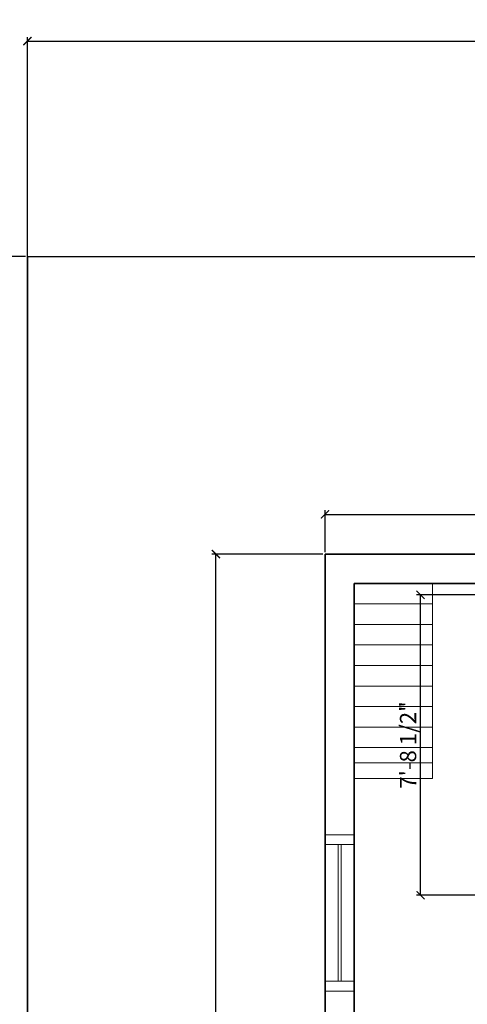
# Model space of a CAD drawing. Units: inches. Extents: x 3283068 to 3284536, y 3240756 to 3241803.
# Tile 8 of 19: x 3283246 to 3283383, y 3241501 to 3241803. Entities that reach past the tile are written whole.
import ezdxf

# ---------------------------------------------------------------- set-up
doc = ezdxf.new("R2010")
doc.units = ezdxf.units.IN
for name, color, linetype, lineweight in [('A-ANNO-DIMS', 2, 'Continuous', 18), ('C-PROP', 7, 'Continuous', 25), ('wall', 20, 'Continuous', 35), ('wardrobe', 180, 'Continuous', 18), ('window', 100, 'Continuous', 18)]:
    doc.layers.add(name, color=color, linetype=linetype, lineweight=lineweight)
doc.styles.get("Standard").update_dxf_attribs({"font": 'arial.ttf'})
doc.dimstyles.new('ISO-25', dxfattribs={"dimtxt": 5, "dimasz": 2.5, "dimexe": 1.25, "dimexo": 0.625, "dimtad": 1, "dimlunit": 4, "dimtxsty": 'Standard', "dimblk": 'ARCHTICK', "dimcen": 2.5, "dimadec": 0, "dimazin": 0, "dimtfac": 1, "dimtmove": 0, "dimatfit": 3, "dimfxl": 1, "dimarcsym": 0})

# ---------------------------------------------------------------- blocks, each defined once
blk = doc.blocks.new('_ArchTick')
at = {"color": 0, "linetype": 'ByBlock', "const_width": 0.15}
blk.add_lwpolyline([(-0.5, -0.5), (0.5, 0.5)], dxfattribs=at)
blk = doc.blocks.new('*D1')
at = {"layer": 'A-ANNO-DIMS', "color": 0, "lineweight": -2, "transparency": 16777216}
for p, q in [((3283338.96, 3241639.1), (3283304.8, 3241639.1)), ((3283306.05, 3241198.1), (3283306.05, 3241639.1)), ((3283338.96, 3241198.1), (3283304.8, 3241198.1))]:
    blk.add_line(p, q, dxfattribs=at)
at = {"layer": 'Defpoints', "color": 0, "transparency": 16777216}
for p in [(3283306.05, 3241639.1), (3283339.59, 3241639.1), (3283339.59, 3241198.1)]:
    blk.add_point(p, dxfattribs=at)
at = {"layer": 'A-ANNO-DIMS', "color": 0, "lineweight": -2, "transparency": 16777216, "xscale": 2.5, "yscale": 2.5, "zscale": 2.5}
for p, rotation in [((3283306.05, 3241639.1), 90), ((3283306.05, 3241198.1), 270)]:
    blk.add_blockref('_ArchTick', p, dxfattribs=dict(at, rotation=rotation))
at = {"layer": 'A-ANNO-DIMS', "color": 0, "transparency": 16777216, "insert": (3283302.87, 3241418.6), "char_height": 5, "attachment_point": 5, "rotation": 90}
blk.add_mtext('36\'-9"', dxfattribs=at)
blk = doc.blocks.new('*D25')
at = {"layer": 'A-ANNO-DIMS', "color": 0, "lineweight": -2, "transparency": 16777216}
for p, q in [((3283339.59, 3241639.73), (3283339.59, 3241652.58)), ((3284236.59, 3241639.73), (3284236.59, 3241652.58)), ((3283339.59, 3241651.33), (3284236.59, 3241651.33))]:
    blk.add_line(p, q, dxfattribs=at)
at = {"layer": 'Defpoints', "color": 0, "transparency": 16777216}
for p in [(3284236.59, 3241651.33), (3283339.59, 3241639.1), (3284236.59, 3241639.1)]:
    blk.add_point(p, dxfattribs=at)
at = {"layer": 'A-ANNO-DIMS', "color": 0, "lineweight": -2, "transparency": 16777216, "xscale": 2.5, "yscale": 2.5, "zscale": 2.5, "rotation": 180}
blk.add_blockref('_ArchTick', (3283339.59, 3241651.33), dxfattribs=at)
at = {"layer": 'A-ANNO-DIMS', "color": 0, "lineweight": -2, "transparency": 16777216, "xscale": 2.5, "yscale": 2.5, "zscale": 2.5}
blk.add_blockref('_ArchTick', (3284236.59, 3241651.33), dxfattribs=at)
at = {"layer": 'A-ANNO-DIMS', "color": 0, "transparency": 16777216, "insert": (3283788.09, 3241654.51), "char_height": 5, "attachment_point": 5}
blk.add_mtext('74\'-9"', dxfattribs=at)
blk = doc.blocks.new('WIN-48IN-9IN-WALL')
for p, q in [((0, 9), (48, 9)), ((0, 0), (0, 9)), ((3, 0), (3, 9)), ((45, 9), (45, 0)), ((48, 9), (48, 0)), ((3, 5), (45, 5)), ((3, 4), (45, 4)), ((48, 0), (0, 0))]:
    blk.add_line(p, q)
blk = doc.blocks.new('WARDROBE-60X24IN')
for p, q in [((0, 53.69), (24, 53.69)), ((0, 47.37), (24, 47.37)), ((0, 41.06), (24, 41.06)), ((0, 34.75), (24, 34.75)), ((0, 28.44), (24, 28.44)), ((0, 22.12), (24, 22.12)), ((0, 15.81), (24, 15.81)), ((0, 9.5), (24, 9.5)), ((0, 4.82), (24, 4.82))]:
    blk.add_line(p, q)
blk.add_lwpolyline([(0, 60), (24, 60), (24, 0), (0, 0)], close=True)
blk = doc.blocks.new('*D58')
at = {"layer": 'A-ANNO-DIMS', "color": 0, "lineweight": -2, "transparency": 16777216}
for p, q in [((3283387.6, 3241626.59), (3283367.72, 3241626.59)), ((3283368.97, 3241534.23), (3283368.97, 3241626.59)), ((3283387.6, 3241534.23), (3283367.72, 3241534.23))]:
    blk.add_line(p, q, dxfattribs=at)
at = {"layer": 'Defpoints', "color": 0, "transparency": 16777216}
for p in [(3283368.97, 3241626.59), (3283388.23, 3241626.59), (3283388.23, 3241534.23)]:
    blk.add_point(p, dxfattribs=at)
at = {"layer": 'A-ANNO-DIMS', "color": 0, "lineweight": -2, "transparency": 16777216, "xscale": 2.5, "yscale": 2.5, "zscale": 2.5}
for p, rotation in [((3283368.97, 3241626.59), 90), ((3283368.97, 3241534.23), 270)]:
    blk.add_blockref('_ArchTick', p, dxfattribs=dict(at, rotation=rotation))
at = {"layer": 'A-ANNO-DIMS', "color": 0, "transparency": 16777216, "insert": (3283365.76, 3241580.41), "char_height": 5, "attachment_point": 5, "rotation": 90}
blk.add_mtext('7\'-8 1/2"', dxfattribs=at)
blk = doc.blocks.new('*D61')
at = {"layer": 'A-ANNO-DIMS', "color": 0, "lineweight": -2, "transparency": 16777216}
for p, q in [((3283247.46, 3241730.6), (3283073.57, 3241730.6)), ((3283074.82, 3241082.6), (3283074.82, 3241730.6)), ((3283247.46, 3241082.6), (3283073.57, 3241082.6))]:
    blk.add_line(p, q, dxfattribs=at)
at = {"layer": 'Defpoints', "color": 0, "transparency": 16777216}
for p in [(3283074.82, 3241730.6), (3283248.09, 3241730.6), (3283248.09, 3241082.6)]:
    blk.add_point(p, dxfattribs=at)
at = {"layer": 'A-ANNO-DIMS', "color": 0, "lineweight": -2, "transparency": 16777216, "xscale": 2.5, "yscale": 2.5, "zscale": 2.5}
for p, rotation in [((3283074.82, 3241730.6), 90), ((3283074.82, 3241082.6), 270)]:
    blk.add_blockref('_ArchTick', p, dxfattribs=dict(at, rotation=rotation))
at = {"layer": 'A-ANNO-DIMS', "color": 0, "transparency": 16777216, "insert": (3283071.64, 3241406.6), "char_height": 5, "attachment_point": 5, "rotation": 90}
blk.add_mtext('54\'-0"', dxfattribs=at)
blk = doc.blocks.new('*D63')
at = {"layer": 'A-ANNO-DIMS', "color": 0, "lineweight": -2, "transparency": 16777216}
for p, q in [((3283248.09, 3241083.23), (3283248.09, 3241798.08)), ((3284328.09, 3241083.23), (3284328.09, 3241798.08)), ((3283248.09, 3241796.83), (3284328.09, 3241796.83))]:
    blk.add_line(p, q, dxfattribs=at)
at = {"layer": 'Defpoints', "color": 0, "transparency": 16777216}
for p in [(3284328.09, 3241796.83), (3283248.09, 3241082.6), (3284328.09, 3241082.6)]:
    blk.add_point(p, dxfattribs=at)
at = {"layer": 'A-ANNO-DIMS', "color": 0, "lineweight": -2, "transparency": 16777216, "xscale": 2.5, "yscale": 2.5, "zscale": 2.5, "rotation": 180}
blk.add_blockref('_ArchTick', (3283248.09, 3241796.83), dxfattribs=at)
at = {"layer": 'A-ANNO-DIMS', "color": 0, "lineweight": -2, "transparency": 16777216, "xscale": 2.5, "yscale": 2.5, "zscale": 2.5}
blk.add_blockref('_ArchTick', (3284328.09, 3241796.83), dxfattribs=at)
at = {"layer": 'A-ANNO-DIMS', "color": 0, "transparency": 16777216, "insert": (3283788.09, 3241800.01), "char_height": 5, "attachment_point": 5}
blk.add_mtext('90\'-0"', dxfattribs=at)

msp = doc.modelspace()

# ---------------------------------------------------------------- linework, layer by layer
at = {"layer": 'C-PROP'}
for q in [(3283248.089, 3241082.602), (3284328.089, 3241730.602)]:
    msp.add_line((3283248.089, 3241730.602), q, dxfattribs=at)
at = {"layer": 'wall'}
for p, q in [((3283339.589, 3241639.102), (3283339.589, 3241198.102)), ((3283339.589, 3241639.102), (3284236.589, 3241639.102)), ((3283348.589, 3241630.102), (3283348.589, 3241496.602)), ((3283348.589, 3241630.102), (3283531.589, 3241630.102))]:
    msp.add_line(p, q, dxfattribs=at)
at = {"layer": 'wardrobe'}
msp.add_line((3283348.589, 3241630.102), (3283372.589, 3241630.102), dxfattribs=at)

# ---------------------------------------------------------------- block references
msp.add_blockref('WARDROBE-60X24IN', (3283348.589, 3241570.102), dxfattribs=at)
at = {"layer": 'window', "rotation": 270.0000000004698}
msp.add_blockref('WIN-48IN-9IN-WALL', (3283339.589, 3241552.773), dxfattribs=at)

# ---------------------------------------------------------------- dimensions: what is measured, and where the dimension line sits
at = {"layer": 'A-ANNO-DIMS'}
for base, p1, p2, override, picture, middle in [((3284328.089, 3241796.827), (3283248.089, 3241082.602), (3284328.089, 3241082.602), {"dimdec": 1, "dimlfac": 1, "dimrnd": 0, "dimzin": 1, "dimdsep": 46, "dimlunit": 4, "dimfrac": 2}, '*D63', (3283788.089, 3241800.005)), ((3284236.589, 3241651.334), (3283339.589, 3241639.102), (3284236.589, 3241639.102), {"dimclrd": 0, "dimclre": 0, "dimclrt": 0}, '*D25', (3283788.089, 3241654.512))]:
    dim = msp.add_linear_dim(base=base, p1=p1, p2=p2, dimstyle='ISO-25', override=override, dxfattribs=at)
    dim.commit()
    dim.dimension.update_dxf_attribs({"geometry": picture, "text_midpoint": middle})
for base, p1, p2, override, picture, middle in [((3283074.817, 3241730.602), (3283248.089, 3241082.602), (3283248.089, 3241730.602), {"dimdec": 1, "dimlfac": 1, "dimrnd": 0, "dimzin": 1, "dimdsep": 46, "dimlunit": 4, "dimfrac": 2}, '*D61', (3283071.639, 3241406.602)), ((3283306.051, 3241639.102), (3283339.589, 3241198.102), (3283339.589, 3241639.102), {"dimclrd": 0, "dimclre": 0, "dimclrt": 0}, '*D1', (3283302.872, 3241418.602)), ((3283368.971, 3241626.59), (3283388.229, 3241534.227), (3283388.229, 3241626.59), {"dimdec": 1, "dimlfac": 1, "dimrnd": 0, "dimzin": 1, "dimdsep": 46, "dimlunit": 4, "dimfrac": 2}, '*D58', (3283365.761, 3241580.409))]:
    dim = msp.add_linear_dim(base=base, p1=p1, p2=p2, angle=90, dimstyle='ISO-25', override=override, dxfattribs=at)
    dim.commit()
    dim.dimension.update_dxf_attribs({"geometry": picture, "text_midpoint": middle})

doc.saveas('drawing.dxf')
